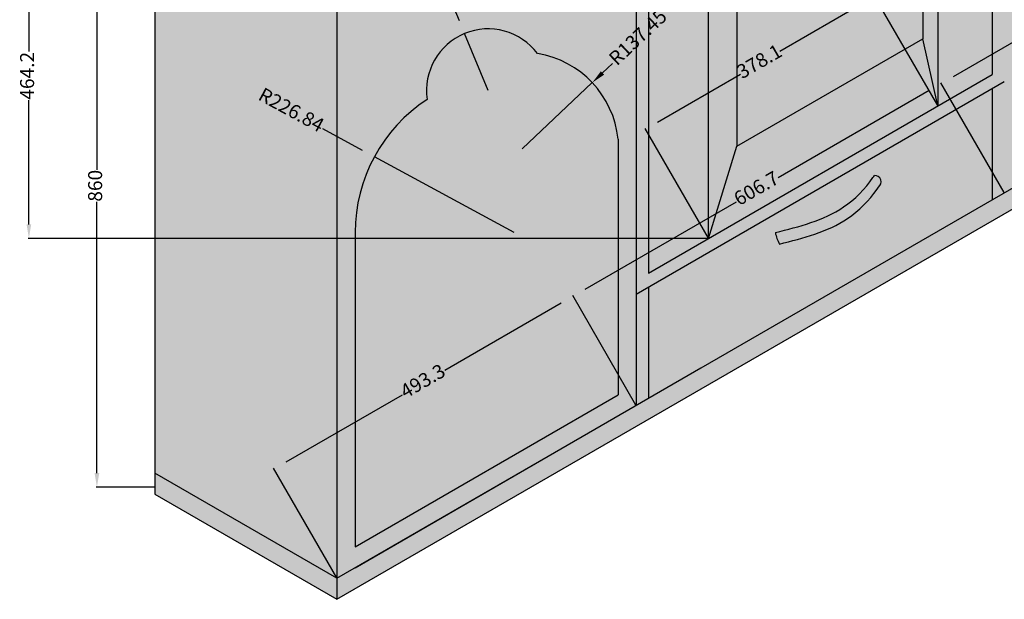
# Model space of a CAD drawing. Units: millimetres. Extents: x 78378 to 86415, y 148682 to 152721.
# Tile 1 of 18: x 78378 to 79783, y 148875 to 149702. Entities that reach past the tile are written whole.
import ezdxf

# ---------------------------------------------------------------- set-up
doc = ezdxf.new("R2010")
doc.units = ezdxf.units.MM
for name, color, linetype, lineweight in [('A-ANNO-DIMS', 2, 'Continuous', 18), ('A-FURN', 4, 'Continuous', 25), ('A-FURN-PATT', 32, 'Continuous', 13)]:
    doc.layers.add(name, color=color, linetype=linetype, lineweight=lineweight)
doc.styles.get("Standard").update_dxf_attribs({"font": 'arial.ttf'})
doc.dimstyles.new('ISO-25', dxfattribs={"dimtxt": 20, "dimasz": 20, "dimexe": 1.25, "dimexo": 0.625, "dimtad": 0, "dimdec": 1, "dimtxsty": 'Standard', "dimcen": 2.5, "dimadec": 0, "dimazin": 0, "dimtfac": 1, "dimtdec": 1, "dimtmove": 0, "dimatfit": 3, "dimfxl": 1, "dimarcsym": 0})

# ---------------------------------------------------------------- blocks, each defined once
blk = doc.blocks.new('*D6')
at = {"layer": 'A-ANNO-DIMS', "color": 0, "lineweight": -2, "transparency": 16777216}
for p, q in [((78570.2, 149895), (78486.7, 149895)), ((78488, 149875), (78488, 149487.7)), ((78488, 149055), (78488, 149442.3)), ((78570.2, 149035), (78486.7, 149035))]:
    blk.add_line(p, q, dxfattribs=at)
at = {"layer": 'A-ANNO-DIMS', "color": 0, "transparency": 16777216}
for points in [[(78484.6, 149875), (78491.3, 149875), (78488, 149895)], [(78484.6, 149055), (78491.3, 149055), (78488, 149035)]]:
    blk.add_solid(points, dxfattribs=at)
at = {"layer": 'Defpoints', "color": 0, "transparency": 16777216}
for p in [(78570.9, 149895), (78488, 149035), (78570.9, 149035)]:
    blk.add_point(p, dxfattribs=at)
at = {"layer": 'A-ANNO-DIMS', "color": 0, "transparency": 16777216, "insert": (78488, 149465), "char_height": 20, "attachment_point": 5, "rotation": 90}
blk.add_mtext('860', dxfattribs=at)
blk = doc.blocks.new('*D20')
at = {"layer": 'A-ANNO-DIMS', "color": 0, "lineweight": -2, "transparency": 16777216}
for p, q in [((79257.5, 149152.2), (79167.2, 149308.6)), ((79150.5, 149297.5), (78984.4, 149201.6)), ((78758, 149070.9), (78924.1, 149166.8)), ((78830.4, 148905.5), (78740, 149062))]:
    blk.add_line(p, q, dxfattribs=at)
at = {"layer": 'A-ANNO-DIMS', "color": 0, "transparency": 16777216}
for points in [[(79148.9, 149300.4), (79152.2, 149294.6), (79167.9, 149307.5)], [(78756.3, 149073.8), (78759.7, 149068), (78740.7, 149060.9)]]:
    blk.add_solid(points, dxfattribs=at)
at = {"layer": 'Defpoints', "color": 0, "transparency": 16777216}
for p in [(79167.9, 149307.5), (79257.9, 149151.6), (78830.7, 148905)]:
    blk.add_point(p, dxfattribs=at)
at = {"layer": 'A-ANNO-DIMS', "color": 0, "transparency": 16777216, "insert": (78954.3, 149184.2), "char_height": 20, "attachment_point": 5, "rotation": 30}
blk.add_mtext('493.3', dxfattribs=at)
blk = doc.blocks.new('*D21')
at = {"layer": 'A-ANNO-DIMS', "color": 0, "lineweight": -2, "transparency": 16777216}
for p, q in [((79783, 149455.5), (79692.7, 149612)), ((79676, 149600.9), (79460.4, 149476.4)), ((79185.2, 149317.5), (79400.8, 149442)), ((79257.5, 149152.2), (79167.2, 149308.6))]:
    blk.add_line(p, q, dxfattribs=at)
at = {"layer": 'A-ANNO-DIMS', "color": 0, "transparency": 16777216}
for points in [[(79674.3, 149603.8), (79677.6, 149598), (79693.3, 149610.9)], [(79183.5, 149320.4), (79186.8, 149314.6), (79167.9, 149307.5)]]:
    blk.add_solid(points, dxfattribs=at)
at = {"layer": 'Defpoints', "color": 0, "transparency": 16777216}
for p in [(79693.3, 149610.9), (79783.3, 149455), (79257.9, 149151.6)]:
    blk.add_point(p, dxfattribs=at)
at = {"layer": 'A-ANNO-DIMS', "color": 0, "transparency": 16777216, "insert": (79430.6, 149459.2), "char_height": 20, "attachment_point": 5, "rotation": 30}
blk.add_mtext('606.7', dxfattribs=at)
blk = doc.blocks.new('*D22')
at = {"layer": 'A-ANNO-DIMS', "color": 0, "lineweight": -2, "transparency": 16777216}
for p, q in [((80086.1, 149630.5), (79995.8, 149787)), ((79979.1, 149775.9), (79864.5, 149709.7)), ((79710.6, 149620.9), (79825.2, 149687.1)), ((79783, 149455.5), (79692.7, 149612))]:
    blk.add_line(p, q, dxfattribs=at)
at = {"layer": 'A-ANNO-DIMS', "color": 0, "transparency": 16777216}
for points in [[(79977.4, 149778.8), (79980.8, 149773), (79996.4, 149785.9)], [(79708.9, 149623.8), (79712.3, 149618), (79693.3, 149610.9)]]:
    blk.add_solid(points, dxfattribs=at)
at = {"layer": 'Defpoints', "color": 0, "transparency": 16777216}
for p in [(79996.4, 149785.9), (80086.4, 149630), (79783.3, 149455)]:
    blk.add_point(p, dxfattribs=at)
at = {"layer": 'A-ANNO-DIMS', "color": 0, "transparency": 16777216, "insert": (79844.8, 149698.4), "char_height": 20, "attachment_point": 5, "rotation": 30}
blk.add_mtext('350', dxfattribs=at)
blk = doc.blocks.new('*D25')
at = {"layer": 'A-ANNO-DIMS', "color": 0, "lineweight": -2, "transparency": 16777216}
for p, q in [((79360.5, 149854), (78389.6, 149854)), ((78390.9, 149834), (78390.9, 149656.6)), ((78390.9, 149409.9), (78390.9, 149587.3)), ((79360.5, 149389.9), (78389.6, 149389.9))]:
    blk.add_line(p, q, dxfattribs=at)
at = {"layer": 'A-ANNO-DIMS', "color": 0, "transparency": 16777216}
for points in [[(78387.5, 149834), (78394.2, 149834), (78390.9, 149854)], [(78387.5, 149409.9), (78394.2, 149409.9), (78390.9, 149389.9)]]:
    blk.add_solid(points, dxfattribs=at)
at = {"layer": 'Defpoints', "color": 0, "transparency": 16777216}
for p in [(78390.9, 149854), (79361.1, 149854), (79361.1, 149389.9)]:
    blk.add_point(p, dxfattribs=at)
at = {"layer": 'A-ANNO-DIMS', "color": 0, "transparency": 16777216, "insert": (78390.9, 149621.9), "char_height": 20, "attachment_point": 5, "rotation": 90}
blk.add_mtext('464.2', dxfattribs=at)
blk = doc.blocks.new('*D26')
at = {"layer": 'A-ANNO-DIMS', "color": 0, "lineweight": -2, "transparency": 16777216}
for p, q in [((79688.2, 149579.5), (79597.9, 149735.9)), ((79581.2, 149724.8), (79462.9, 149656.5)), ((79288.4, 149555.7), (79406.7, 149624.1)), ((79360.8, 149390.4), (79270.5, 149546.8))]:
    blk.add_line(p, q, dxfattribs=at)
at = {"layer": 'A-ANNO-DIMS', "color": 0, "transparency": 16777216}
for points in [[(79579.6, 149727.7), (79582.9, 149721.9), (79598.5, 149734.8)], [(79286.8, 149558.6), (79290.1, 149552.9), (79271.1, 149545.7)]]:
    blk.add_solid(points, dxfattribs=at)
at = {"layer": 'Defpoints', "color": 0, "transparency": 16777216}
for p in [(79598.5, 149734.8), (79688.5, 149578.9), (79361.1, 149389.9)]:
    blk.add_point(p, dxfattribs=at)
at = {"layer": 'A-ANNO-DIMS', "color": 0, "transparency": 16777216, "insert": (79434.8, 149640.3), "char_height": 20, "attachment_point": 5, "rotation": 30}
blk.add_mtext('378.1', dxfattribs=at)
blk = doc.blocks.new('*D60')
at = {"layer": 'A-ANNO-DIMS', "color": 0, "lineweight": -2, "transparency": 16777216}
for p, q in [((78809.8, 149546.5), (78866.4, 149515.8)), ((79083.5, 149398.3), (78884, 149506.3))]:
    blk.add_line(p, q, dxfattribs=at)
at = {"layer": 'A-ANNO-DIMS', "color": 0, "transparency": 16777216}
blk.add_solid([(78868, 149518.8), (78864.9, 149512.9), (78884, 149506.3)], dxfattribs=at)
at = {"layer": 'Defpoints', "color": 0, "transparency": 16777216}
for p in [(78884, 149506.3), (79083.5, 149398.3)]:
    blk.add_point(p, dxfattribs=at)
at = {"layer": 'A-ANNO-DIMS', "color": 0, "transparency": 16777216, "insert": (78764.4, 149571.1), "char_height": 20, "attachment_point": 5, "rotation": 331.5585}
blk.add_mtext('R226.84', dxfattribs=at)
blk = doc.blocks.new('*D61')
at = {"layer": 'A-ANNO-DIMS', "color": 0, "lineweight": -2, "transparency": 16777216}
for p, q in [((79224.2, 149639.6), (79209.7, 149625.9)), ((79095.1, 149517.9), (79195.1, 149612.1))]:
    blk.add_line(p, q, dxfattribs=at)
at = {"layer": 'A-ANNO-DIMS', "color": 0, "transparency": 16777216}
blk.add_solid([(79207.4, 149628.3), (79212, 149623.4), (79195.1, 149612.1)], dxfattribs=at)
at = {"layer": 'Defpoints', "color": 0, "transparency": 16777216}
for p in [(79195.1, 149612.1), (79095.1, 149517.9)]:
    blk.add_point(p, dxfattribs=at)
at = {"layer": 'A-ANNO-DIMS', "color": 0, "transparency": 16777216, "insert": (79261.9, 149675.1), "char_height": 20, "attachment_point": 5, "rotation": 43.3062}
blk.add_mtext('R137.45', dxfattribs=at)
blk = doc.blocks.new('*D62')
at = {"layer": 'A-ANNO-DIMS', "color": 0, "lineweight": -2, "transparency": 16777216}
for p, q in [((78997.4, 149719), (79005.1, 149700.6)), ((79046.5, 149600.8), (79012.8, 149682.1))]:
    blk.add_line(p, q, dxfattribs=at)
at = {"layer": 'A-ANNO-DIMS', "color": 0, "transparency": 16777216}
blk.add_solid([(79008.2, 149701.8), (79002, 149699.3), (79012.8, 149682.1)], dxfattribs=at)
at = {"layer": 'Defpoints', "color": 0, "transparency": 16777216}
for p in [(79012.8, 149682.1), (79046.5, 149600.8)]:
    blk.add_point(p, dxfattribs=at)
at = {"layer": 'A-ANNO-DIMS', "color": 0, "transparency": 16777216, "insert": (78988, 149741.7), "char_height": 20, "attachment_point": 5, "rotation": 292.5474}
blk.add_mtext('R88', dxfattribs=at)

msp = doc.modelspace()

# ---------------------------------------------------------------- hatches: boundary and pattern name
at = {"layer": 'A-FURN-PATT'}
h = msp.add_hatch(color=256, dxfattribs=at)
h.dxf.hatch_style = 1
h.paths.add_polyline_path([(79765.9748, 149445.0076), (79765.9748, 149603.6184), (79275.1761, 149320.2556), (79275.1761, 149161.6449), (79350.2826, 149205.0076)])
edge = h.paths.add_edge_path(flags=16)
edge.add_arc((79507.244, 149406.7325), 51.4573, 189.4892034, 208.9818028, ccw=False)
edge.add_spline(control_points=[(79456.4908, 149398.2492), (79490.7805, 149406.8496), (79544.6682, 149420.3656), (79585.6167, 149461.099), (79597.2078, 149478.6257), (79597.8866, 149479.6521)], knot_values=[0, 0, 0, 0, 103.871151751, 163.238054653, 166.930945274, 166.930945274, 166.930945274, 166.930945274], degree=3, periodic=0)
edge.add_arc((79598.468, 149470.6289), 9.0419, -55.2157026, 93.6867088, ccw=False)
edge.add_spline(control_points=[(79603.6263, 149463.2027), (79602.9475, 149462.1763), (79591.3564, 149444.6496), (79550.4079, 149403.9163), (79496.5202, 149390.4003), (79462.2305, 149381.7998)], knot_values=[0, 0, 0, 0, 3.692890621, 63.059793523, 166.930945274, 166.930945274, 166.930945274, 166.930945274], degree=3, periodic=0)
h.paths.add_polyline_path([(80060.4234, 149980.8221), (80060.4234, 150256.6366), (79809.2761, 150111.6366), (79809.2761, 149835.8221)], flags=0)
edge = h.paths.add_edge_path(flags=0)
edge.add_arc((79897.9874, 150103.5556), 5.1726, 122.0794663, 231.0916039, ccw=False)
edge.add_spline(control_points=[(79895.2403, 150107.9384), (79905.0476, 150110.9384), (79924.6357, 150116.9304), (79948.7961, 150128.9973), (79958.1258, 150141.8088), (79961.3514, 150146.2382)], knot_values=[0, 0, 0, 0, 30.92804237, 61.772539507, 78.071660491, 78.071660491, 78.071660491, 78.071660491], degree=3, periodic=0)
edge.add_arc((79956.2102, 150141.1519), 7.232, -40.6762437, 44.6926573, ccw=False)
edge.add_spline(control_points=[(79961.695, 150136.4382), (79958.1075, 150132.5465), (79947.5299, 150121.0716), (79924.3289, 150108.3481), (79904.611, 150102.4724), (79894.7387, 150099.5306)], knot_values=[0, 0, 0, 0, 15.829606447, 46.674103584, 77.602145954, 77.602145954, 77.602145954, 77.602145954], degree=3, periodic=0)
h.paths.add_polyline_path([(80060.4234, 149950.8221), (79809.2761, 149805.8221), (79809.2761, 149500.0076), (80060.4234, 149645.0076)], flags=0)
edge = h.paths.add_edge_path(flags=0)
edge.add_arc((79897.9874, 149795.6302), 5.1726, 122.0794663, 231.0916039, ccw=False)
edge.add_spline(control_points=[(79895.2403, 149800.013), (79905.0476, 149803.013), (79924.6357, 149809.005), (79948.7961, 149821.0719), (79958.1258, 149833.8834), (79961.3514, 149838.3128)], knot_values=[0, 0, 0, 0, 30.92804237, 61.772539507, 78.071660491, 78.071660491, 78.071660491, 78.071660491], degree=3, periodic=0)
edge.add_arc((79956.2102, 149833.2265), 7.232, -40.6762437, 44.6926573, ccw=False)
edge.add_spline(control_points=[(79961.695, 149828.5129), (79958.1075, 149824.6211), (79947.5299, 149813.1462), (79924.3289, 149800.4227), (79904.611, 149794.547), (79894.7387, 149791.6052)], knot_values=[0, 0, 0, 0, 15.829606447, 46.674103584, 77.602145954, 77.602145954, 77.602145954, 77.602145954], degree=3, periodic=0)
h.paths.add_polyline_path([(80086.4042, 150301.6366), (79783.2953, 150126.6366), (79783.2953, 149455.0076), (80086.4042, 149630.0076)])
h.paths.add_polyline_path([(79809.2761, 150111.6366), (80060.4234, 150256.6366), (80060.4234, 149980.8221), (79809.2761, 149835.8221)], flags=16)
h.paths.add_polyline_path([(80060.4234, 149950.8221), (80060.4234, 149645.0076), (79809.2761, 149500.0076), (79809.2761, 149805.8221)], flags=16)
h = msp.add_hatch(color=256, dxfattribs=at)
h.dxf.hatch_style = 1
h.paths.add_polyline_path([(79765.9748, 150214.3024), (79275.1761, 149930.9396), (79275.1761, 149340.2556), (79361.1019, 149389.8649), (79361.1019, 149854.0252), (79688.5392, 150043.0712), (79688.5392, 149578.9109), (79765.9748, 149623.6184)], flags=0)
h.paths.add_polyline_path([(79616.9975, 150064.3358, -1), (79579.5778, 150064.3358, -1)], flags=0)
h.paths.add_polyline_path([(79511.257, 150003.2865, -1), (79473.8373, 150003.2865, -1)], flags=0)
h.paths.add_polyline_path([(79398.6146, 149938.2524, -1), (79361.1949, 149938.2524, -1)], flags=0)
h.paths.add_polyline_path([(79688.5392, 149578.9109), (79667.1607, 149674.8368), (79401.2524, 149521.3146), (79361.1019, 149389.8649)], flags=0)
h.paths.add_polyline_path([(79783.2953, 149613.6184), (79783.2953, 150126.6366), (79783.2953, 150265.0076), (79257.8556, 149961.6449), (79257.8556, 149310.2556)])
h.paths.add_polyline_path([(79275.1761, 149340.2556), (79275.1761, 149930.9396), (79765.9748, 150214.3024), (79765.9748, 149623.6184)], flags=16)
h.paths.add_polyline_path([(79361.1019, 149389.8649), (79361.1019, 149854.0252), (79688.5392, 150043.0712), (79688.5392, 149578.9109), (79667.1607, 149674.8368), (79401.2524, 149521.3146)], flags=0)
h.paths.add_polyline_path([(79477.9029, 149864.6773), (79477.9029, 149877.6076), (79571.7852, 149931.8105), (79571.7852, 149918.8803)], flags=0)
h = msp.add_hatch(color=256, dxfattribs=at)
h.dxf.hatch_style = 1
h.set_gradient(color1=(39, 118, 187), color2=(122, 175, 223))
h.paths.add_polyline_path([(79667.1607, 149961.6903), (79401.2524, 149808.168), (79401.2524, 149521.3146), (79667.1607, 149674.8368)], flags=17)
h.paths.add_polyline_path([(79765.9748, 150214.3024), (79275.1761, 149930.9396), (79275.1761, 149340.2556), (79361.1019, 149389.8649), (79361.1019, 149854.0252), (79688.5392, 150043.0712), (79688.5392, 149578.9109), (79765.9748, 149623.6184)])
h.paths.add_polyline_path([(79579.5778, 150064.3358, -1), (79616.9975, 150064.3358, -1)], flags=16)
h.paths.add_polyline_path([(79511.257, 150003.2865, -1), (79473.8373, 150003.2865, -1)], flags=16)
h.paths.add_polyline_path([(79398.6146, 149938.2524, -1), (79361.1949, 149938.2524, -1)], flags=16)
h = msp.add_hatch(color=256, dxfattribs=at)
h.dxf.hatch_style = 1
h.paths.add_polyline_path([(81125.6347, 150190.0076), (81116.9744, 150195.0076), (81116.9744, 149762.4135), (81125.6347, 149757.4135)])
h.paths.add_polyline_path([(81125.6347, 149757.4135), (81116.9744, 149762.4135), (81116.9744, 149732.4135), (81125.6347, 149727.4135)])
h.paths.add_polyline_path([(79275.1761, 149320.2556), (79257.8556, 149310.2556), (79257.8556, 149151.6449), (79275.1761, 149161.6449)])
h.paths.add_polyline_path([(79783.2953, 149613.6184), (79765.9748, 149603.6184), (79765.9748, 149445.0076), (79783.2953, 149455.0076)])
h.paths.add_polyline_path([(79765.9748, 149445.0076), (79765.9748, 149603.6184), (79275.1761, 149320.2556), (79275.1761, 149161.6449), (79350.2826, 149205.0076)])
edge = h.paths.add_edge_path(flags=0)
edge.add_spline(control_points=[(79456.4908, 149398.2492), (79490.7805, 149406.8496), (79544.6682, 149420.3656), (79585.6167, 149461.099), (79597.2078, 149478.6257), (79597.8866, 149479.6521)], knot_values=[0, 0, 0, 0, 103.871151751, 163.238054653, 166.930945274, 166.930945274, 166.930945274, 166.930945274], degree=3, periodic=0)
edge.add_arc((79598.468, 149470.6289), 9.0419, -55.2157026, 93.6867088, ccw=False)
edge.add_spline(control_points=[(79603.6263, 149463.2027), (79602.9475, 149462.1763), (79591.3564, 149444.6496), (79550.4079, 149403.9163), (79496.5202, 149390.4003), (79462.2305, 149381.7998)], knot_values=[0, 0, 0, 0, 3.692890621, 63.059793523, 166.930945274, 166.930945274, 166.930945274, 166.930945274], degree=3, periodic=0)
edge.add_arc((79507.244, 149406.7325), 51.4573, 189.4892034, 208.9818028, ccw=False)
edge = h.paths.add_edge_path(flags=16)
edge.add_spline(control_points=[(79462.2305, 149381.7998), (79496.5202, 149390.4003), (79550.4079, 149403.9163), (79591.3564, 149444.6496), (79602.9475, 149462.1763), (79603.6263, 149463.2027)], knot_values=[0, 0, 0, 0, 103.871151751, 163.238054653, 166.930945274, 166.930945274, 166.930945274, 166.930945274], degree=3, periodic=0)
edge.add_arc((79598.468, 149470.6289), 9.0419, 304.7842974, 453.6867088)
edge.add_spline(control_points=[(79597.8866, 149479.6521), (79597.2078, 149478.6257), (79585.6167, 149461.099), (79544.6682, 149420.3656), (79490.7805, 149406.8496), (79456.4908, 149398.2492)], knot_values=[0, 0, 0, 0, 3.692890621, 63.059793523, 166.930945274, 166.930945274, 166.930945274, 166.930945274], degree=3, periodic=0)
edge.add_arc((79507.244, 149406.7325), 51.4573, 189.4892034, 208.9818028)
h = msp.add_hatch(color=256, dxfattribs=at)
h.dxf.hatch_style = 1
h.paths.add_polyline_path([(79401.2524, 149808.168), (79361.1019, 149854.0252), (79361.1019, 149389.8649), (79401.2524, 149521.3146)])
h.paths.add_polyline_path([(79667.1607, 149961.6903), (79688.5392, 150043.0712), (79361.1019, 149854.0252), (79401.2524, 149808.168)])
h.paths.add_polyline_path([(79477.9029, 149864.6773), (79477.9029, 149877.6076), (79571.7852, 149931.8105), (79571.7852, 149918.8803)], flags=16)
h.paths.add_polyline_path([(79688.5392, 150043.0712), (79667.1607, 149961.6903), (79667.1607, 149674.8368), (79688.5392, 149578.9109)])
h = msp.add_hatch(color=256, dxfattribs=at)
h.dxf.hatch_style = 1
h.paths.add_polyline_path([(78830.6674, 149715.0076), (78570.8597, 149865.0076), (78570.8597, 149055.0076), (78830.6674, 148905.0076)])
h.paths.add_polyline_path([(79257.8556, 149981.6449), (78830.6674, 149735.0076), (78830.6674, 148905.0076), (79257.8556, 149151.6449)])
h.paths.add_polyline_path([(79116.9453, 149653.5787, -0.339994387), (79231.8748, 149531.6449), (79231.8748, 149166.6449), (78856.6481, 148950.0076), (78856.6481, 149398.1143, -0.253423643), (78959.4208, 149588.1766, -0.777144535)], flags=16)
h.paths.add_polyline_path([(79231.8748, 149531.6449, 0.339994387), (79116.9453, 149653.5787, 0.777144535), (78959.4208, 149588.1766, 0.253423643), (78856.6481, 149398.1143), (78856.6481, 148950.0076), (79231.8748, 149166.6449)], flags=0)
h = msp.add_hatch(color=256, dxfattribs=at)
h.dxf.hatch_style = 1
h.paths.add_polyline_path([(79231.8748, 149531.6449, 0.339994387), (79116.9453, 149653.5787, 0.777144535), (78959.4208, 149588.1766, 0.253423643), (78856.6481, 149398.1143), (78856.6481, 148950.0076), (79231.8748, 149166.6449)])
h = msp.add_hatch(color=256, dxfattribs=at)
h.dxf.hatch_style = 1
h.paths.add_polyline_path([(79667.1607, 149674.8368), (79401.2524, 149521.3146), (79361.1019, 149389.8649), (79688.5392, 149578.9109)])
h = msp.add_hatch(color=256, dxfattribs=at)
h.dxf.hatch_style = 1
h.paths.add_polyline_path([(80086.4042, 149600.0076), (80692.622, 149584.0076), (81239.9694, 149267.9965), (81239.9694, 149297.9965), (81116.9744, 149369.0076), (80692.622, 149614.0076), (80086.4042, 149630.0076), (78830.6674, 148905.0076), (78830.6674, 148875.0076)])
h = msp.add_hatch(color=256, dxfattribs=at)
h.dxf.hatch_style = 1
edge = h.paths.add_edge_path()
edge.add_spline(control_points=[(79462.2305, 149381.7998), (79496.5202, 149390.4003), (79550.4079, 149403.9163), (79591.3564, 149444.6496), (79602.9475, 149462.1763), (79603.6263, 149463.2027)], knot_values=[0, 0, 0, 0, 103.871151751, 163.238054653, 166.930945274, 166.930945274, 166.930945274, 166.930945274], degree=3, periodic=0)
edge.add_arc((79598.468, 149470.6289), 9.0419, 304.7842974, 453.6867088)
edge.add_spline(control_points=[(79597.8866, 149479.6521), (79597.2078, 149478.6257), (79585.6167, 149461.099), (79544.6682, 149420.3656), (79490.7805, 149406.8496), (79456.4908, 149398.2492)], knot_values=[0, 0, 0, 0, 3.692890621, 63.059793523, 166.930945274, 166.930945274, 166.930945274, 166.930945274], degree=3, periodic=0)
edge.add_arc((79507.244, 149406.7325), 51.4573, 189.4892034, 208.9818028)
h = msp.add_hatch(color=256, dxfattribs=at)
h.dxf.hatch_style = 1
h.paths.add_polyline_path([(78570.8597, 149055.0076), (78570.8597, 149025.0076), (78830.6674, 148875.0076), (78830.6674, 148905.0076)])

# ---------------------------------------------------------------- linework, layer by layer
at = {"layer": 'A-FURN'}
for p, q in [((79765.9748, 150214.3024), (79765.9748, 149623.6184)), ((79688.5392, 150043.0712), (79688.5392, 149578.9109)), ((79257.8556, 149981.6449), (79257.8556, 149151.6449)), ((79667.1607, 149961.6903), (79667.1607, 149674.8368)), ((79275.1761, 149930.9396), (79275.1761, 149340.2556)), ((78570.8597, 149885.0076), (78570.8597, 149025.0076)), ((79361.1019, 149389.8649), (79361.1019, 149854.0252)), ((79401.2524, 149808.168), (79401.2524, 149521.3146)), ((78830.6674, 149735.0076), (78830.6674, 148875.0076)), ((79401.2524, 149521.3146), (79667.1607, 149674.8368)), ((79688.5392, 149578.9109), (79667.1607, 149674.8368)), ((78830.6674, 148905.0076), (80086.4042, 149630.0076)), ((79275.1761, 149340.2556), (79765.9748, 149623.6184)), ((79257.8556, 149310.2556), (79783.2953, 149613.6184)), ((78830.6674, 148875.0076), (80086.4042, 149600.0076)), ((79765.9748, 149603.6184), (79765.9748, 149445.0076)), ((79231.8748, 149531.6449), (79231.8748, 149166.6449)), ((79361.1019, 149389.8649), (79401.2524, 149521.3146)), ((78856.6481, 149398.4305), (78856.6481, 148950.0076)), ((79275.1761, 149320.2556), (79275.1761, 149161.6449)), ((78856.6481, 148920.0076), (79350.2826, 149205.0076)), ((78856.6481, 148950.0076), (79231.8748, 149166.6449)), ((78830.6674, 148905.0076), (78570.8597, 149055.0076)), ((78570.8597, 149025.0076), (78830.6674, 148875.0076))]:
    msp.add_line(p, q, dxfattribs=at)
for centre, radius, start, end in [((79046.5156, 149600.8083), 88.006, 36.842864, 188.2523446), ((79095.1156, 149517.8722), 137.451, 5.7507047, 80.8616844), ((79083.4875, 149398.2724), 226.8394, 123.1570667, 179.9600706), ((79598.468, 149470.6289), 9.0419, 304.7842974, 93.6867088), ((79507.244, 149406.7325), 51.4573, 189.4892034, 208.9818028)]:
    msp.add_arc(centre, radius, start, end, dxfattribs=at)
for points in [[(79456.4908, 149398.2492), (79490.7805, 149406.8496), (79544.6682, 149420.3656), (79585.6167, 149461.099), (79597.2078, 149478.6257), (79597.8866, 149479.6521)], [(79462.2305, 149381.7998), (79496.5202, 149390.4003), (79550.4079, 149403.9163), (79591.3564, 149444.6496), (79602.9475, 149462.1763), (79603.6263, 149463.2027)]]:
    msp.add_open_spline(points, degree=3, knots=[0, 0, 0, 0, 103.871151751, 163.238054653, 166.930945274, 166.930945274, 166.930945274, 166.930945274], dxfattribs=at)

# ---------------------------------------------------------------- dimensions: what is measured, and where the dimension line sits
at = {"layer": 'A-ANNO-DIMS'}
dim = msp.add_aligned_dim(p1=(78570.8597, 149895.0076), p2=(78570.8597, 149035.0076), distance=-82.8905, dimstyle='ISO-25', override={"dimclrd": 0, "dimclre": 0, "dimclrt": 0}, dxfattribs=at)
dim.commit()
dim.dimension.update_dxf_attribs({"geometry": '*D6', "text_midpoint": (78487.9692, 149465.0076)})
for base, p1, p2, angle, override, picture, middle in [((78390.8597, 149854.0252), (79361.1019, 149389.8649), (79361.1019, 149854.0252), 90, {"dimdec": 1, "dimlfac": 1, "dimrnd": 0, "dimzin": 0, "dimdsep": 46, "dimlunit": 2}, '*D25', (78390.8597, 149621.945)), ((79996.4042, 149785.8922), (79783.2953, 149455.0076), (80086.4042, 149630.0076), 30, {"dimdec": 0, "dimlfac": 1, "dimrnd": 0, "dimzin": 0, "dimdsep": 46, "dimlunit": 2}, '*D22', (79844.8498, 149698.3922)), ((79598.5392, 149734.7955), (79361.1019, 149389.8649), (79688.5392, 149578.9109), 30, {"dimdec": 1, "dimlfac": 1, "dimrnd": 0, "dimzin": 0, "dimdsep": 46, "dimlunit": 2}, '*D26', (79434.8205, 149640.2725)), ((79693.2953, 149610.8922), (79257.8556, 149151.6449), (79783.2953, 149455.0076), 30, {"dimdec": 1, "dimlfac": 1, "dimrnd": 0, "dimzin": 0, "dimdsep": 46, "dimlunit": 2}, '*D21', (79430.5755, 149459.2108)), ((79167.8556, 149307.5295), (78830.6674, 148905.0076), (79257.8556, 149151.6449), 30, {"dimdec": 1, "dimlfac": 1, "dimrnd": 0, "dimzin": 0, "dimdsep": 46, "dimlunit": 2}, '*D20', (78954.2615, 149184.2108))]:
    dim = msp.add_linear_dim(base=base, p1=p1, p2=p2, angle=angle, dimstyle='ISO-25', override=override, dxfattribs=at)
    dim.commit()
    dim.dimension.update_dxf_attribs({"geometry": picture, "text_midpoint": middle})
for center, mpoint, override, picture, middle in [((79046.5156, 149600.8083), (79012.7698, 149682.0874), {"dimdec": 0, "dimlfac": 1, "dimrnd": 0, "dimzin": 0, "dimdsep": 46, "dimlunit": 2}, '*D62', (78988.0219, 149741.6945)), ((79095.1156, 149517.8722), (79195.1385, 149612.1495), {"dimdec": 2, "dimlfac": 1, "dimrnd": 0, "dimzin": 0, "dimdsep": 46, "dimlunit": 2}, '*D61', (79261.9301, 149675.1043))]:
    dim = msp.add_radius_dim(center=center, mpoint=mpoint, dimstyle='ISO-25', override=override, dxfattribs=at)
    dim.commit()
    dim.dimension.update_dxf_attribs({"geometry": picture, "text_midpoint": middle})
dim = msp.add_radius_dim(center=(79083.4875, 149398.2724), mpoint=(78884.0267, 149506.3072), dimstyle='ISO-25', override={"dimdec": 2, "dimlfac": 1, "dimrnd": 0, "dimzin": 0, "dimdsep": 46, "dimlunit": 2}, dxfattribs=at)
dim.commit()
dim.dimension.update_dxf_attribs({"geometry": '*D60', "text_midpoint": (78764.3502, 149571.128), "dimtype": 164})

doc.saveas('drawing.dxf')
